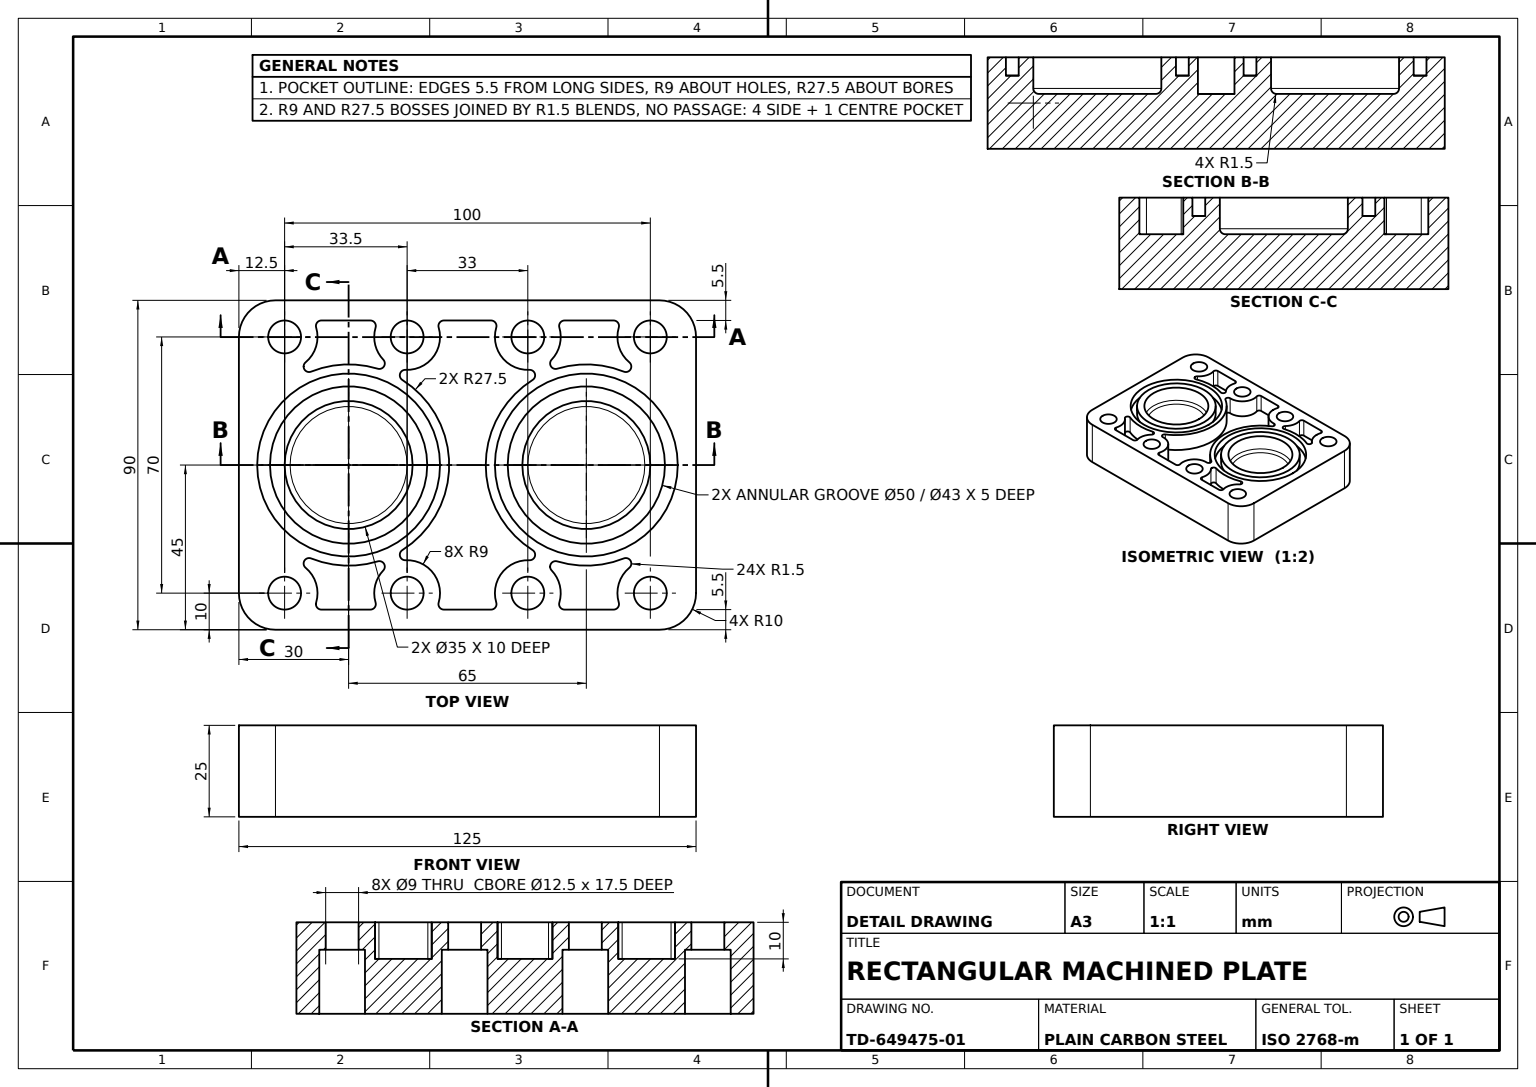
from build123d import *

# Parameters (mm, degrees)
BLOCK_PROFILE_SKETCH_W         = 125
BLOCK_PROFILE_SKETCH_H         = 25
BASE_BLOCK_DEPTH               = 45
BORE_RECESS_SKETCH_R           = 25
BORE_RECESS_SKETCH_R_2         = 21.5
BORE_RECESS_5MM_DEPTH          = 5
TWIN_BORE_SKETCH_R             = 17.5
TWIN_BORES_DEPTH               = 10
BORE_EDGE_FILLET_R1_5_R        = 1.5
RELIEF_POCKETS_DEPTH           = 10
BOLT_HOLES_CBORE_9_D           = 9
BOLT_HOLES_CBORE_9_DEPTH       = 100
BOLT_HOLES_CBORE_9_CBORE_D     = 12.5
BOLT_HOLES_CBORE_9_CBORE_DEPTH = 17.5
CORNER_FILLETS_R10_R           = 10


with BuildPart() as part:
    # Block Profile Sketch → Base Block (new, symmetric)
    with BuildSketch(Plane(origin=(0, 0, 0), x_dir=(0, 0, -1), z_dir=(1, 0, 0))):
        Rectangle(BLOCK_PROFILE_SKETCH_W, BLOCK_PROFILE_SKETCH_H)
    extrude(amount=BASE_BLOCK_DEPTH, both=True)

    # Bore Recess Sketch → Bore Recess 5mm (cut)
    # profile 1 of 2: a face of its own
    with BuildSketch(Plane(origin=(0, 12.5, 0), x_dir=(1, 0, 0), z_dir=(0, 1, 0))):
        with Locations(Location((0, 32.5, 0), (0, 0, 270))):
            Circle(BORE_RECESS_SKETCH_R)
        with Locations(Location((0, 32.5, 0), (0, 0, 270))):
            Circle(BORE_RECESS_SKETCH_R_2, mode=Mode.SUBTRACT)
    # profile 2 of 2: a face of its own
    with BuildSketch(Plane(origin=(0, 12.5, 0), x_dir=(1, 0, 0), z_dir=(0, 1, 0))):
        with Locations(Location((0, -32.5, 0), (0, 0, 90))):
            Circle(BORE_RECESS_SKETCH_R)
        with Locations(Location((0, -32.5, 0), (0, 0, 90))):
            Circle(BORE_RECESS_SKETCH_R_2, mode=Mode.SUBTRACT)
    extrude(amount=-BORE_RECESS_5MM_DEPTH, mode=Mode.SUBTRACT)

    # Twin Bore Sketch → Twin Bores (cut)
    with BuildSketch(Plane(origin=(0, 12.5, 0), x_dir=(1, 0, 0), z_dir=(0, 1, 0))):
        with Locations(Location((0, 32.5, 0), (0, 0, 270))):
            Circle(TWIN_BORE_SKETCH_R)
        with Locations(Location((0, -32.5, 0), (0, 0, 270))):
            Circle(TWIN_BORE_SKETCH_R)
    extrude(amount=-TWIN_BORES_DEPTH, mode=Mode.SUBTRACT)

    # Bore Edge Fillet R1.5
    bore_edge_fillet_r1_5_edges = [part.edges().sort_by_distance(p)[0] for p in [
        (0, 2.5, -50),
        (0, 2.5, 15),
    ]]
    fillet(bore_edge_fillet_r1_5_edges, radius=BORE_EDGE_FILLET_R1_5_R)

    # Relief Pocket Sketch → Relief Pockets (cut)
    with BuildSketch(Plane(origin=(0, 12.5, 0), x_dir=(1, 0, 0), z_dir=(0, 1, 0))):
        with BuildLine():
            Line((-39.5, 6.437694101), (-39.5, -6.437694101))
            ThreePointArc((-39.5, -6.437694101), (-38.896421457, -7.64036969), (-37.571428571, -7.875166373))
            ThreePointArc((-37.571428571, -7.875166373), (-29.450149328, -9.41486362), (-26.010329741, -16.931078451))
            ThreePointArc((-26.010329741, -16.931078451), (-24.963701576, -18.433313648), (-23.244186639, -17.804497711))
            ThreePointArc((-23.244186639, -17.804497711), (0, -5), (23.244186639, -17.804497711))
            ThreePointArc((23.244186639, -17.804497711), (24.963701576, -18.433313648), (26.010329741, -16.931078451))
            ThreePointArc((26.010329741, -16.931078451), (29.450149328, -9.41486362), (37.571428571, -7.875166373))
            ThreePointArc((37.571428571, -7.875166373), (38.896421457, -7.64036969), (39.5, -6.437694101))
            Line((39.5, -6.437694101), (39.5, 6.437694101))
            ThreePointArc((39.5, 6.437694101), (38.896421457, 7.64036969), (37.571428571, 7.875166373))
            ThreePointArc((37.571428571, 7.875166373), (29.450149328, 9.41486362), (26.010329741, 16.931078451))
            ThreePointArc((26.010329741, 16.931078451), (24.963701576, 18.433313648), (23.244186639, 17.804497711))
            ThreePointArc((23.244186639, 17.804497711), (0, 5), (-23.244186639, 17.804497711))
            ThreePointArc((-23.244186639, 17.804497711), (-24.963701576, 18.433313648), (-26.010329741, 16.931078451))
            ThreePointArc((-26.010329741, 16.931078451), (-29.450149328, 9.41486362), (-37.571428571, 7.875166373))
            ThreePointArc((-37.571428571, 7.875166373), (-38.896421457, 7.64036969), (-39.5, 6.437694101))
        make_face()
        with BuildLine():
            Line((-39.5, -26.562305899), (-39.5, -39.937694101))
            ThreePointArc((-39.5, -39.937694101), (-38.896421457, -41.14036969), (-37.571428571, -41.375166373))
            ThreePointArc((-37.571428571, -41.375166373), (-32.385666254, -41.388074602), (-28.067872341, -44.260173686))
            ThreePointArc((-28.067872341, -44.260173686), (-26.145612251, -44.5926659), (-25.520490952, -42.744732383))
            ThreePointArc((-25.520490952, -42.744732383), (-27.473408366, -33.709062761), (-26.321795689, -24.53676751))
            ThreePointArc((-26.321795689, -24.53676751), (-26.971313668, -22.824965098), (-28.792168571, -23.016350892))
            ThreePointArc((-28.792168571, -23.016350892), (-32.898267073, -25.251155278), (-37.571428571, -25.124833627))
            ThreePointArc((-37.571428571, -25.124833627), (-38.896421457, -25.35963031), (-39.5, -26.562305899))
        make_face()
        with BuildLine():
            Line((-39.5, 39.937694101), (-39.5, 26.562305899))
            ThreePointArc((-39.5, 26.562305899), (-38.896421457, 25.35963031), (-37.571428571, 25.124833627))
            ThreePointArc((-37.571428571, 25.124833627), (-32.898267073, 25.251155278), (-28.792168571, 23.016350892))
            ThreePointArc((-28.792168571, 23.016350892), (-26.971313668, 22.824965098), (-26.321795689, 24.53676751))
            ThreePointArc((-26.321795689, 24.53676751), (-27.473408366, 33.709062761), (-25.520490952, 42.744732383))
            ThreePointArc((-25.520490952, 42.744732383), (-26.145612251, 44.5926659), (-28.067872341, 44.260173686))
            ThreePointArc((-28.067872341, 44.260173686), (-32.385666254, 41.388074602), (-37.571428571, 41.375166373))
            ThreePointArc((-37.571428571, 41.375166373), (-38.896421457, 41.14036969), (-39.5, 39.937694101))
        make_face()
        with BuildLine():
            Line((39.5, -26.562305899), (39.5, -39.937694101))
            ThreePointArc((39.5, -39.937694101), (38.896421457, -41.14036969), (37.571428571, -41.375166373))
            ThreePointArc((37.571428571, -41.375166373), (32.385666254, -41.388074602), (28.067872341, -44.260173686))
            ThreePointArc((28.067872341, -44.260173686), (26.145612251, -44.5926659), (25.520490952, -42.744732383))
            ThreePointArc((25.520490952, -42.744732383), (27.473408366, -33.709062761), (26.321795689, -24.53676751))
            ThreePointArc((26.321795689, -24.53676751), (26.971313668, -22.824965098), (28.792168571, -23.016350892))
            ThreePointArc((28.792168571, -23.016350892), (32.898267073, -25.251155278), (37.571428571, -25.124833627))
            ThreePointArc((37.571428571, -25.124833627), (38.896421457, -25.35963031), (39.5, -26.562305899))
        make_face()
        with BuildLine():
            Line((39.5, 39.937694101), (39.5, 26.562305899))
            ThreePointArc((39.5, 26.562305899), (38.896421457, 25.35963031), (37.571428571, 25.124833627))
            ThreePointArc((37.571428571, 25.124833627), (32.898267073, 25.251155278), (28.792168571, 23.016350892))
            ThreePointArc((28.792168571, 23.016350892), (26.971313668, 22.824965098), (26.321795689, 24.53676751))
            ThreePointArc((26.321795689, 24.53676751), (27.473408366, 33.709062761), (25.520490952, 42.744732383))
            ThreePointArc((25.520490952, 42.744732383), (26.145612251, 44.5926659), (28.067872341, 44.260173686))
            ThreePointArc((28.067872341, 44.260173686), (32.385666254, 41.388074602), (37.571428571, 41.375166373))
            ThreePointArc((37.571428571, 41.375166373), (38.896421457, 41.14036969), (39.5, 39.937694101))
        make_face()
    extrude(amount=-RELIEF_POCKETS_DEPTH, mode=Mode.SUBTRACT)

    # Bolt Holes CBore Ø9
    with Locations(Plane(origin=(0, -12.5, 0), x_dir=(-1, 0, 0), z_dir=(0, -1, 0))):
        with Locations((-35, -50), (35, -50), (-35, -16.5), (-35, 16.5), (-35, 50), (35, 50), (35, 16.5), (35, -16.5)):
            CounterBoreHole(BOLT_HOLES_CBORE_9_D / 2, BOLT_HOLES_CBORE_9_CBORE_D / 2, BOLT_HOLES_CBORE_9_CBORE_DEPTH, depth=BOLT_HOLES_CBORE_9_DEPTH)

    # Corner Fillets R10
    corner_fillets_r10_edges = [part.edges().sort_by_distance(p)[0] for p in [
        (45, 0, 62.5),
        (45, 0, -62.5),
        (-45, 0, 62.5),
        (-45, 0, -62.5),
    ]]
    fillet(corner_fillets_r10_edges, radius=CORNER_FILLETS_R10_R)


solid = part.part
